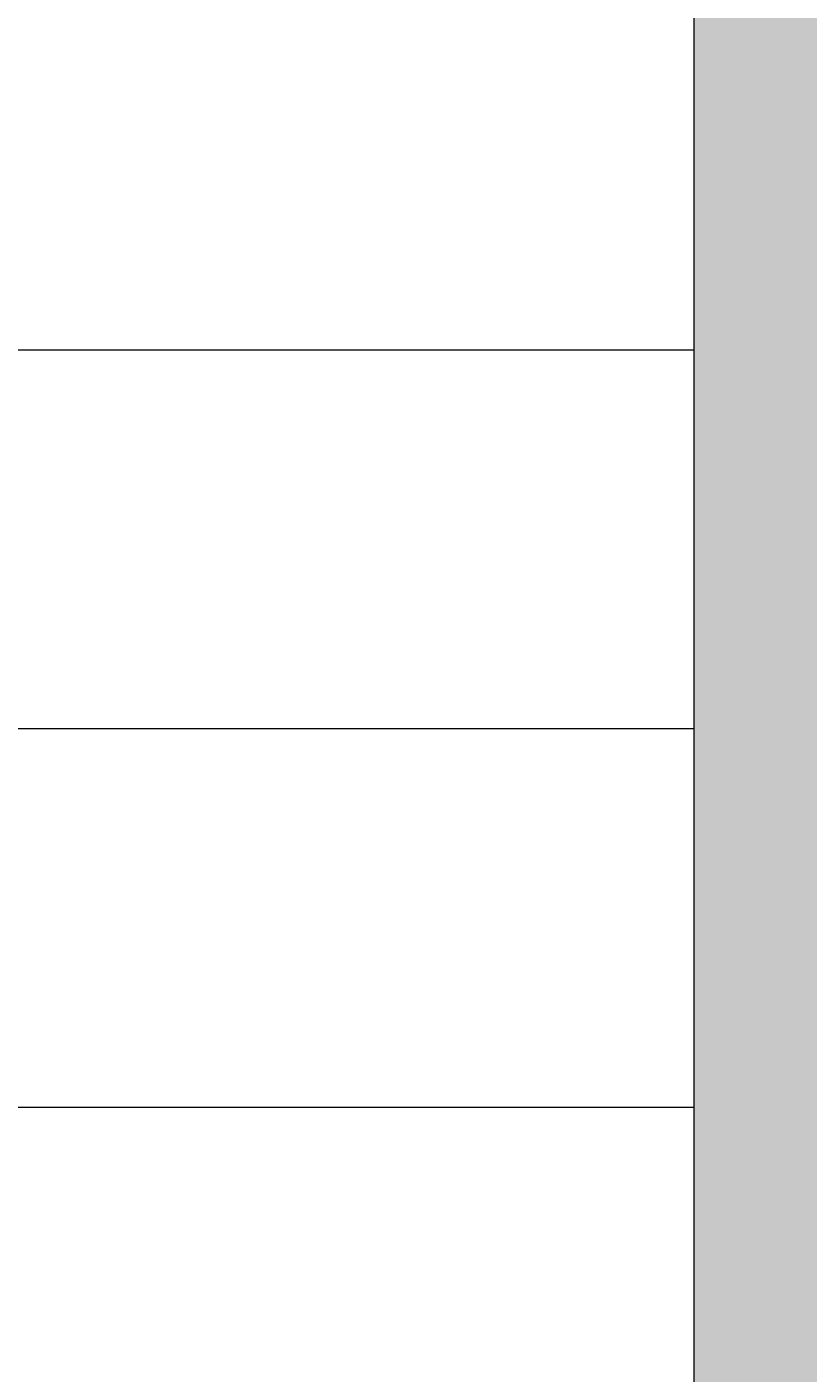
# Model space of a CAD drawing. Units: inches. Extents: x 84 to 1044, y -280 to 906.
# Tile 56 of 105: x 374.88 to 387.99, y 738.5 to 761.07. Entities that reach past the tile are written whole.
import ezdxf

# ---------------------------------------------------------------- set-up
doc = ezdxf.new("R2010")
doc.units = ezdxf.units.IN
doc.layers.add('A-ANNO-DIMS', color=2, linetype='Continuous', lineweight=18)
doc.layers.add('L-HRDS', color=32, linetype='Continuous', lineweight=18)
doc.layers.add('A-FLOR-PATT', color=251, linetype='Continuous', lineweight=9, true_color=0x705861)
doc.layers.add('L-PLNT-PATT', color=9, linetype='Continuous', lineweight=9, true_color=0xafd9aa)
doc.styles.get("Standard").update_dxf_attribs({"font": 'arial.ttf'})
doc.dimstyles.get("Standard").update_dxf_attribs({"dimtxt": 0.18, "dimasz": 0.18, "dimexe": 0.18, "dimexo": 0.0625, "dimgap": 0.09, "dimtad": 0, "dimtih": 1, "dimtoh": 1, "dimdec": 4, "dimzin": 0, "dimdsep": 46, "dimtxsty": 'Standard', "dimcen": 0.09, "dimadec": 0, "dimazin": 0, "dimtfac": 1, "dimtdec": 4, "dimtofl": 0, "dimtmove": 0, "dimatfit": 3, "dimfxl": 1, "dimtolj": 1, "dimtzin": 0, "dimarcsym": 0})

# ---------------------------------------------------------------- blocks, each defined once
blk = doc.blocks.new('*D62')
at = {"layer": 'A-ANNO-DIMS', "color": 0, "lineweight": -2, "transparency": 16777216}
for p, q in [((203.179, 709.183), (203.179, 905.9)), ((896.074, 400.183), (896.074, 905.9)), ((203.359, 905.72), (549.232, 905.72)), ((895.894, 905.72), (550.021, 905.72))]:
    blk.add_line(p, q, dxfattribs=at)
at = {"layer": 'A-ANNO-DIMS', "color": 0, "transparency": 16777216}
for points in [[(203.359, 905.75), (203.359, 905.69), (203.179, 905.72)], [(895.894, 905.75), (895.894, 905.69), (896.074, 905.72)]]:
    blk.add_solid(points, dxfattribs=at)
at = {"layer": 'Defpoints', "color": 0, "transparency": 16777216}
for p in [(896.074, 905.72), (203.179, 709.12), (896.074, 400.12)]:
    blk.add_point(p, dxfattribs=at)
at = {"layer": 'A-ANNO-DIMS', "color": 0, "transparency": 16777216, "insert": (549.627, 905.72), "char_height": 0.18, "attachment_point": 5}
blk.add_mtext('\\A1;692.9', dxfattribs=at)

msp = doc.modelspace()

# ---------------------------------------------------------------- hatches: boundary and pattern name
at = {"layer": 'A-FLOR-PATT', "transparency": 33554597}
h = msp.add_hatch(dxfattribs=at)
h.set_pattern_fill('DOLMIT', color=256)
h.paths.add_polyline_path([(896.074, 709.12), (833.074, 709.12), (833.074, 646.12), (833.074, 574.12), (833.074, 511.12), (896.074, 511.12)])
h.paths.add_polyline_path([(386.074, 769.12), (203.179, 769.12), (203.179, 709.12), (287.127, 709.12), (359.127, 709.12), (386.074, 709.12)])
at = {"layer": 'L-PLNT-PATT', "transparency": 33554597}
h = msp.add_hatch(color=256, dxfattribs=at)
h.dxf.hatch_style = 1
h.paths.add_polyline_path([(434.074, 769.12), (386.074, 769.12), (386.074, 709.12), (434.074, 709.12)])
h.paths.add_polyline_path([(896.074, 847.12), (434.074, 847.12), (434.074, 769.12), (434.074, 709.12), (470.074, 709.12), (506.074, 709.12), (572.074, 709.12), (608.074, 709.12), (698.074, 709.12), (770.074, 709.12), (833.074, 709.12), (896.074, 709.12)])
h.paths.add_polyline_path([(983.074, 847.12), (896.074, 847.12), (896.074, 709.12), (896.074, 547.12), (932.074, 547.12), (983.074, 547.12)])
h.paths.add_polyline_path([(983.074, 547.12), (932.074, 547.12), (932.074, 265.12), (983.074, 265.12)])
h.paths.add_polyline_path([(203.179, 646.12), (203.179, 709.12), (203.179, 745.12), (143.179, 745.12), (143.179, 271.12), (203.179, 271.12), (203.179, 274.12), (203.179, 310.12), (203.179, 574.12)])

# ---------------------------------------------------------------- linework, layer by layer
at = {"layer": 'L-HRDS'}
msp.add_line((386.074, 769.12), (386.074, 709.12), dxfattribs=at)

# ---------------------------------------------------------------- dimensions: what is measured, and where the dimension line sits
at = {"layer": 'A-ANNO-DIMS'}
dim = msp.add_linear_dim(base=(896.074, 905.72), p1=(203.179, 709.12), p2=(896.074, 400.12), dimstyle='Standard', override={"dimdec": 1, "dimlfac": 1, "dimrnd": 0, "dimzin": 0, "dimdsep": 46, "dimlunit": 2}, dxfattribs=at)
dim.commit()
dim.dimension.update_dxf_attribs({"geometry": '*D62', "text_midpoint": (549.627, 905.72)})

doc.saveas('drawing.dxf')
